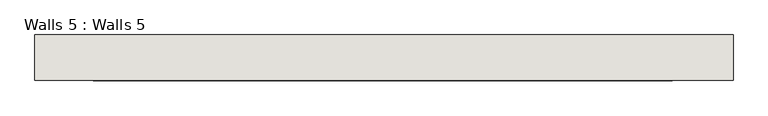
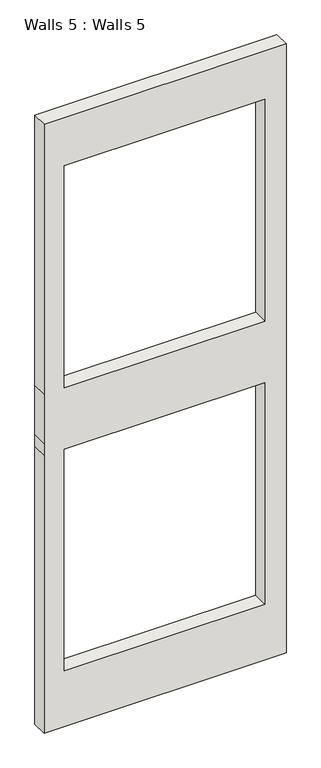
"""IFC4 building model written with IfcOpenShell, lengths in millimetres: wall geometry, Walls 5 : Walls 5."""

from ifc_helpers import new_model, si_unit, frame, origin, place, context, project, spatial, polyline, outline, extrude, source, transform, mapped, element, save


def walls_5_walls_5_f65b2cef(model_context):
    return source(origin(), model_context, "Body", "SweptSolid", [
        extrude(outline(polyline([(12990.5535049, 1357.5254876), (12990.5535049, -2489.4459973), (8449.8316285, -2489.4459973), (7623.0321664, -2489.4459973), (7417.334706, -2489.4459973), (2756.732239, -2489.4459973), (2756.732239, 1357.5254876), (7417.334706, 1357.5254876), (8468.8816285, 1357.5254876), (12990.5535049, 1357.5254876)]), holes=[polyline([(12177.2816285, 1020.9754876), (8449.8316285, 1020.9754876), (8449.8316285, -2166.7245124), (12177.2816285, -2166.7245124), (12177.2816285, 1020.9754876)]), polyline([(3689.884706, -2166.7245124), (7417.334706, -2166.7245124), (7417.334706, 1020.9754876), (3689.884706, 1020.9754876), (3689.884706, -2166.7245124)])]), frame((0.0, -1135.4051517, 0.0), z_axis=(0.0, 1.0, 0.0), x_axis=(0.0, 0.0, 1.0)), (0.0, 0.0, 1.0), 250.6660999),
    ])


if __name__ == "__main__":
    model = new_model("IFC4")
    model_context = context("Model", 3, world=origin())
    ifc_project = project(units=[si_unit("LENGTHUNIT", "METRE", prefix="MILLI")], contexts=[model_context])
    site = spatial("IfcSite", under=ifc_project)
    building = spatial("IfcBuilding", under=site)
    placement = place(None, origin())
    walls_5_walls_5_shape = walls_5_walls_5_f65b2cef(model_context)
    element("IfcWall", 1, ObjectType="Walls 5 : Walls 5", at=placement, inside=building, context=model_context, shape_type="MappedRepresentation", body=[
        mapped(walls_5_walls_5_shape, transform((0.0, 0.0, 0.0), x_axis=(1.0, 0.0, 0.0), y_axis=(0.0, 1.0, 0.0), z_axis=(0.0, 0.0, 1.0))),
    ])
    save(model, "model.ifc")

# Revit data of these elements
# Element 1 (IfcWall, "Walls 5 : Walls 5")
#   Materials on its faces: "Default Wall"
# Materials
#   "Default Wall": colour RGB 128 128 128, transparency 0
